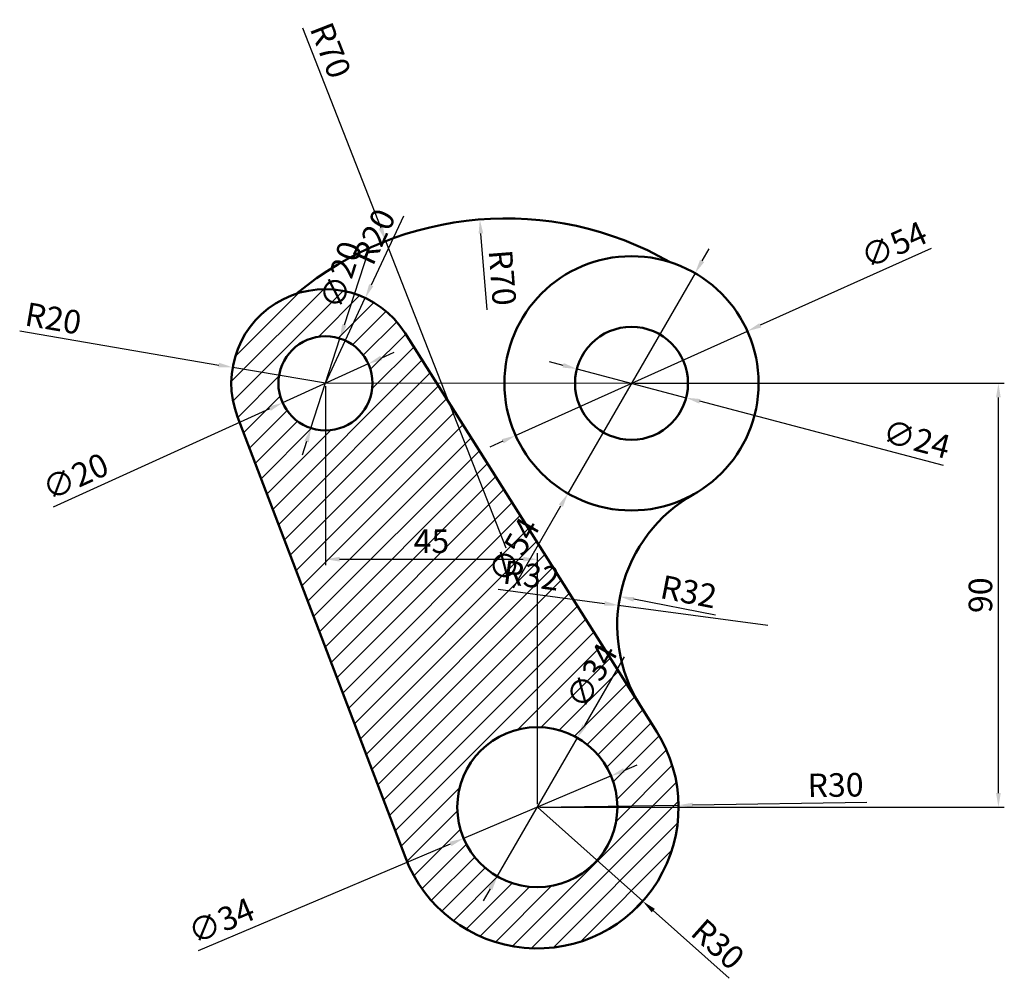
# Model space of a CAD drawing. Units: millimetres. Extents: x 2614 to 2823, y 1450 to 1654.
import ezdxf

# ---------------------------------------------------------------- set-up
doc = ezdxf.new("R2010")
doc.units = ezdxf.units.MM
for name, color, linetype, lineweight in [('M-CONS', 8, 'Continuous', 13), ('M-DIMS', 2, 'Continuous', 25), ('M-HATC', 252, 'Continuous', 18), ('M-OUTL', 7, 'Continuous', 50)]:
    doc.layers.add(name, color=color, linetype=linetype, lineweight=lineweight)
doc.styles.get("Standard").update_dxf_attribs({"font": 'arial.ttf'})
doc.dimstyles.new('ISO-25', dxfattribs={"dimtxt": 5, "dimasz": 3, "dimexe": 1.25, "dimexo": 0.625, "dimtad": 1, "dimtxsty": 'Standard', "dimcen": 3, "dimadec": 0, "dimazin": 0, "dimtfac": 1, "dimtmove": 0, "dimatfit": 3, "dimfxl": 1, "dimarcsym": 0})

# ---------------------------------------------------------------- blocks, each defined once
blk = doc.blocks.new('*D1')
at = {"layer": 'Defpoints', "color": 0, "transparency": 16777216}
for p in [(2739.77, 1493.26), (2708.46, 1480.01)]:
    blk.add_point(p, dxfattribs=at)
at = {"layer": 'M-DIMS', "color": 0, "lineweight": -2, "transparency": 16777216}
for p, q in [((2742.54, 1494.43), (2745.3, 1495.6)), ((2739.77, 1493.26), (2708.46, 1480.01)), ((2652.15, 1456.18), (2705.7, 1478.84))]:
    blk.add_line(p, q, dxfattribs=at)
at = {"layer": 'M-DIMS', "color": 0, "transparency": 16777216}
for points in [[(2742.34, 1494.89), (2742.73, 1493.97), (2739.77, 1493.26)], [(2705.5, 1479.3), (2705.89, 1478.38), (2708.46, 1480.01)]]:
    blk.add_solid(points, dxfattribs=at)
at = {"layer": 'M-DIMS', "color": 0, "transparency": 16777216, "insert": (2657.22, 1461.93), "char_height": 5, "attachment_point": 5, "rotation": 22.939}
blk.add_mtext('∅34', dxfattribs=at)
blk = doc.blocks.new('*D2')
at = {"layer": 'Defpoints', "color": 0, "transparency": 16777216}
for p in [(2688.22, 1580.77), (2670.01, 1572.5)]:
    blk.add_point(p, dxfattribs=at)
at = {"layer": 'M-DIMS', "color": 0, "lineweight": -2, "transparency": 16777216}
for p, q in [((2690.95, 1582.01), (2693.68, 1583.26)), ((2688.22, 1580.77), (2670.01, 1572.5)), ((2621.35, 1550.38), (2667.28, 1571.26))]:
    blk.add_line(p, q, dxfattribs=at)
at = {"layer": 'M-DIMS', "color": 0, "transparency": 16777216}
for points in [[(2690.75, 1582.47), (2691.16, 1581.56), (2688.22, 1580.77)], [(2667.08, 1571.71), (2667.49, 1570.8), (2670.01, 1572.5)]]:
    blk.add_solid(points, dxfattribs=at)
at = {"layer": 'M-DIMS', "color": 0, "transparency": 16777216, "insert": (2626.27, 1556.26), "char_height": 5, "attachment_point": 5, "rotation": 24.4406}
blk.add_mtext('∅20', dxfattribs=at)
blk = doc.blocks.new('*D3')
at = {"layer": 'Defpoints', "color": 0, "transparency": 16777216}
for p in [(2768.74, 1587.72), (2719.5, 1565.55)]:
    blk.add_point(p, dxfattribs=at)
at = {"layer": 'M-DIMS', "color": 0, "lineweight": -2, "transparency": 16777216}
for p, q in [((2807.78, 1605.29), (2771.48, 1588.95)), ((2719.5, 1565.55), (2768.74, 1587.72)), ((2716.76, 1564.32), (2714.02, 1563.09))]:
    blk.add_line(p, q, dxfattribs=at)
at = {"layer": 'M-DIMS', "color": 0, "transparency": 16777216}
for points in [[(2771.27, 1589.4), (2771.68, 1588.49), (2768.74, 1587.72)], [(2716.56, 1564.78), (2716.97, 1563.87), (2719.5, 1565.55)]]:
    blk.add_solid(points, dxfattribs=at)
at = {"layer": 'M-DIMS', "color": 0, "transparency": 16777216, "insert": (2800.11, 1605.47), "char_height": 5, "attachment_point": 5, "rotation": 24.2297}
blk.add_mtext('∅54', dxfattribs=at)
blk = doc.blocks.new('*D4')
at = {"layer": 'Defpoints', "color": 0, "transparency": 16777216}
for p in [(2732.51, 1579.69), (2755.72, 1573.58)]:
    blk.add_point(p, dxfattribs=at)
at = {"layer": 'M-DIMS', "color": 0, "lineweight": -2, "transparency": 16777216}
for p, q in [((2729.61, 1580.45), (2726.71, 1581.22)), ((2732.51, 1579.69), (2755.72, 1573.58)), ((2810.37, 1559.19), (2758.62, 1572.82))]:
    blk.add_line(p, q, dxfattribs=at)
at = {"layer": 'M-DIMS', "color": 0, "transparency": 16777216}
for points in [[(2729.74, 1580.94), (2729.48, 1579.97), (2732.51, 1579.69)], [(2758.75, 1573.3), (2758.5, 1572.33), (2755.72, 1573.58)]]:
    blk.add_solid(points, dxfattribs=at)
at = {"layer": 'M-DIMS', "color": 0, "transparency": 16777216, "insert": (2804.52, 1564.16), "char_height": 5, "attachment_point": 5, "rotation": 345.2499}
blk.add_mtext('∅24', dxfattribs=at)
blk = doc.blocks.new('*D5')
at = {"layer": 'Defpoints', "color": 0, "transparency": 16777216}
for p in [(2754.11, 1487.05), (2724.12, 1486.64)]:
    blk.add_point(p, dxfattribs=at)
at = {"layer": 'M-DIMS', "color": 0, "lineweight": -2, "transparency": 16777216}
for p, q in [((2724.12, 1486.64), (2754.11, 1487.05)), ((2794.1, 1487.6), (2757.11, 1487.09))]:
    blk.add_line(p, q, dxfattribs=at)
at = {"layer": 'M-DIMS', "color": 0, "transparency": 16777216}
blk.add_solid([(2757.11, 1487.59), (2757.12, 1486.59), (2754.11, 1487.05)], dxfattribs=at)
at = {"layer": 'M-DIMS', "color": 0, "transparency": 16777216, "insert": (2787.47, 1490.69), "char_height": 5, "attachment_point": 5, "rotation": 0.7936}
blk.add_mtext('R30', dxfattribs=at)
blk = doc.blocks.new('*D6')
at = {"layer": 'Defpoints', "color": 0, "transparency": 16777216}
for p in [(2659.41, 1580.02), (2679.12, 1576.64)]:
    blk.add_point(p, dxfattribs=at)
at = {"layer": 'M-DIMS', "color": 0, "lineweight": -2, "transparency": 16777216}
for p, q in [((2614.17, 1587.77), (2656.45, 1580.52)), ((2679.12, 1576.64), (2659.41, 1580.02))]:
    blk.add_line(p, q, dxfattribs=at)
at = {"layer": 'M-DIMS', "color": 0, "transparency": 16777216}
blk.add_solid([(2656.53, 1581.01), (2656.36, 1580.03), (2659.41, 1580.02)], dxfattribs=at)
at = {"layer": 'M-DIMS', "color": 0, "transparency": 16777216, "insert": (2621.2, 1589.79), "char_height": 5, "attachment_point": 5, "rotation": 350.2703}
blk.add_mtext('R20', dxfattribs=at)
blk = doc.blocks.new('*D7')
at = {"layer": 'Defpoints', "color": 0, "transparency": 16777216}
for p in [(2711.9, 1611.43), (2717.47, 1541.65)]:
    blk.add_point(p, dxfattribs=at)
at = {"layer": 'M-DIMS', "color": 0, "lineweight": -2, "transparency": 16777216}
blk.add_line((2713.43, 1592.21), (2712.14, 1608.44), dxfattribs=at)
at = {"layer": 'M-DIMS', "color": 0, "transparency": 16777216}
blk.add_solid([(2712.63, 1608.48), (2711.64, 1608.4), (2711.9, 1611.43)], dxfattribs=at)
at = {"layer": 'M-DIMS', "color": 0, "transparency": 16777216, "insert": (2716.07, 1599.03), "char_height": 5, "attachment_point": 5, "rotation": 274.5634}
blk.add_mtext('R70', dxfattribs=at)
blk = doc.blocks.new('*D8')
at = {"layer": 'Defpoints', "color": 0, "transparency": 16777216}
for p in [(2741.66, 1531.34), (2773.07, 1525.23)]:
    blk.add_point(p, dxfattribs=at)
at = {"layer": 'M-DIMS', "color": 0, "lineweight": -2, "transparency": 16777216}
blk.add_line((2761.99, 1527.39), (2744.61, 1530.77), dxfattribs=at)
at = {"layer": 'M-DIMS', "color": 0, "transparency": 16777216}
blk.add_solid([(2744.7, 1531.26), (2744.51, 1530.27), (2741.66, 1531.34)], dxfattribs=at)
at = {"layer": 'M-DIMS', "color": 0, "transparency": 16777216, "insert": (2756.14, 1531.76), "char_height": 5, "attachment_point": 5, "rotation": 348.9946}
blk.add_mtext('R32', dxfattribs=at)
blk = doc.blocks.new('*D9')
at = {"layer": 'Defpoints', "color": 0, "transparency": 16777216}
for p in [(2744.12, 1576.64), (2822.05, 1576.64), (2724.12, 1486.64)]:
    blk.add_point(p, dxfattribs=at)
at = {"layer": 'M-DIMS', "color": 0, "lineweight": -2, "transparency": 16777216}
for p, q in [((2744.74, 1576.64), (2823.3, 1576.64)), ((2822.05, 1489.64), (2822.05, 1573.64)), ((2724.74, 1486.64), (2823.3, 1486.64))]:
    blk.add_line(p, q, dxfattribs=at)
at = {"layer": 'M-DIMS', "color": 0, "transparency": 16777216}
for points in [[(2821.55, 1573.64), (2822.55, 1573.64), (2822.05, 1576.64)], [(2821.55, 1489.64), (2822.55, 1489.64), (2822.05, 1486.64)]]:
    blk.add_solid(points, dxfattribs=at)
at = {"layer": 'M-DIMS', "color": 0, "transparency": 16777216, "insert": (2818.88, 1531.64), "char_height": 5, "attachment_point": 5, "rotation": 90}
blk.add_mtext('90', dxfattribs=at)
blk = doc.blocks.new('*D10')
at = {"layer": 'Defpoints', "color": 0, "transparency": 16777216}
for p in [(2679.12, 1576.64), (2724.12, 1539.29), (2724.12, 1486.64)]:
    blk.add_point(p, dxfattribs=at)
at = {"layer": 'M-DIMS', "color": 0, "lineweight": -2, "transparency": 16777216}
for p, q in [((2679.12, 1576.01), (2679.12, 1538.04)), ((2682.12, 1539.29), (2721.12, 1539.29)), ((2724.12, 1487.26), (2724.12, 1540.54))]:
    blk.add_line(p, q, dxfattribs=at)
at = {"layer": 'M-DIMS', "color": 0, "transparency": 16777216}
for points in [[(2682.12, 1539.79), (2682.12, 1538.79), (2679.12, 1539.29)], [(2721.12, 1539.79), (2721.12, 1538.79), (2724.12, 1539.29)]]:
    blk.add_solid(points, dxfattribs=at)
at = {"layer": 'M-DIMS', "color": 0, "transparency": 16777216, "insert": (2701.62, 1542.46), "char_height": 5, "attachment_point": 5}
blk.add_mtext('45', dxfattribs=at)
blk = doc.blocks.new('*D11')
at = {"layer": 'Defpoints', "color": 0, "transparency": 16777216}
for p in [(2691.96, 1606.84), (2717.47, 1541.65)]:
    blk.add_point(p, dxfattribs=at)
at = {"layer": 'M-DIMS', "color": 0, "lineweight": -2, "transparency": 16777216}
for p, q in [((2674.26, 1652.09), (2690.87, 1609.63)), ((2717.47, 1541.65), (2691.96, 1606.84))]:
    blk.add_line(p, q, dxfattribs=at)
at = {"layer": 'M-DIMS', "color": 0, "transparency": 16777216}
blk.add_solid([(2691.34, 1609.82), (2690.4, 1609.45), (2691.96, 1606.84)], dxfattribs=at)
at = {"layer": 'M-DIMS', "color": 0, "transparency": 16777216, "insert": (2679.62, 1647.11), "char_height": 5, "attachment_point": 5, "rotation": 291.3666}
blk.add_mtext('R70', dxfattribs=at)
blk = doc.blocks.new('*D12')
at = {"layer": 'Defpoints', "color": 0, "transparency": 16777216}
for p in [(2724.12, 1486.64), (2746.51, 1466.67)]:
    blk.add_point(p, dxfattribs=at)
at = {"layer": 'M-DIMS', "color": 0, "lineweight": -2, "transparency": 16777216}
for p, q in [((2724.12, 1486.64), (2746.51, 1466.67)), ((2764.86, 1450.3), (2748.74, 1464.67))]:
    blk.add_line(p, q, dxfattribs=at)
at = {"layer": 'M-DIMS', "color": 0, "transparency": 16777216}
blk.add_solid([(2749.08, 1465.04), (2748.41, 1464.3), (2746.51, 1466.67)], dxfattribs=at)
at = {"layer": 'M-DIMS', "color": 0, "transparency": 16777216, "insert": (2762.05, 1457.06), "char_height": 5, "attachment_point": 5, "rotation": 318.2667}
blk.add_mtext('R30', dxfattribs=at)
blk = doc.blocks.new('*D13')
at = {"layer": 'Defpoints', "color": 0, "transparency": 16777216}
for p in [(2757.62, 1600.02), (2730.62, 1553.25)]:
    blk.add_point(p, dxfattribs=at)
at = {"layer": 'M-DIMS', "color": 0, "lineweight": -2, "transparency": 16777216}
for p, q in [((2759.12, 1602.62), (2760.62, 1605.21)), ((2757.62, 1600.02), (2730.62, 1553.25)), ((2719.06, 1533.23), (2729.12, 1550.65))]:
    blk.add_line(p, q, dxfattribs=at)
at = {"layer": 'M-DIMS', "color": 0, "transparency": 16777216}
for points in [[(2758.68, 1602.87), (2759.55, 1602.37), (2757.62, 1600.02)], [(2728.69, 1550.9), (2729.55, 1550.4), (2730.62, 1553.25)]]:
    blk.add_solid(points, dxfattribs=at)
at = {"layer": 'M-DIMS', "color": 0, "transparency": 16777216, "insert": (2719.65, 1540.88), "char_height": 5, "attachment_point": 5, "rotation": 60.0007}
blk.add_mtext('∅54', dxfattribs=at)
blk = doc.blocks.new('*D14')
at = {"layer": 'Defpoints', "color": 0, "transparency": 16777216}
for p in [(2687.57, 1594.76), (2679.12, 1576.64)]:
    blk.add_point(p, dxfattribs=at)
at = {"layer": 'M-DIMS', "color": 0, "lineweight": -2, "transparency": 16777216}
for p, q in [((2695.68, 1612.14), (2688.84, 1597.48)), ((2679.12, 1576.64), (2687.57, 1594.76))]:
    blk.add_line(p, q, dxfattribs=at)
at = {"layer": 'M-DIMS', "color": 0, "transparency": 16777216}
blk.add_solid([(2688.39, 1597.69), (2689.29, 1597.27), (2687.57, 1594.76)], dxfattribs=at)
at = {"layer": 'M-DIMS', "color": 0, "transparency": 16777216, "insert": (2690.01, 1607.51), "char_height": 5, "attachment_point": 5, "rotation": 64.999}
blk.add_mtext('R20', dxfattribs=at)
blk = doc.blocks.new('*D15')
at = {"layer": 'Defpoints', "color": 0, "transparency": 16777216}
for p in [(2732.62, 1501.36), (2715.62, 1471.91)]:
    blk.add_point(p, dxfattribs=at)
at = {"layer": 'M-DIMS', "color": 0, "lineweight": -2, "transparency": 16777216}
for p, q in [((2742.53, 1518.53), (2734.12, 1503.96)), ((2715.62, 1471.91), (2732.62, 1501.36)), ((2714.12, 1469.31), (2712.62, 1466.72))]:
    blk.add_line(p, q, dxfattribs=at)
at = {"layer": 'M-DIMS', "color": 0, "transparency": 16777216}
for points in [[(2733.69, 1504.21), (2734.55, 1503.71), (2732.62, 1501.36)], [(2713.68, 1469.56), (2714.55, 1469.06), (2715.62, 1471.91)]]:
    blk.add_solid(points, dxfattribs=at)
at = {"layer": 'M-DIMS', "color": 0, "transparency": 16777216, "insert": (2736.2, 1514.2), "char_height": 5, "attachment_point": 5, "rotation": 59.9979}
blk.add_mtext('∅34', dxfattribs=at)
blk = doc.blocks.new('*D16')
at = {"layer": 'Defpoints', "color": 0, "transparency": 16777216}
for p in [(2682.2, 1586.15), (2676.04, 1567.12)]:
    blk.add_point(p, dxfattribs=at)
at = {"layer": 'M-DIMS', "color": 0, "lineweight": -2, "transparency": 16777216}
for p, q in [((2688.31, 1605.02), (2683.12, 1589)), ((2676.04, 1567.12), (2682.2, 1586.15)), ((2675.11, 1564.27), (2674.19, 1561.41))]:
    blk.add_line(p, q, dxfattribs=at)
at = {"layer": 'M-DIMS', "color": 0, "transparency": 16777216}
for points in [[(2682.65, 1589.16), (2683.6, 1588.85), (2682.2, 1586.15)], [(2674.64, 1564.42), (2675.59, 1564.11), (2676.04, 1567.12)]]:
    blk.add_solid(points, dxfattribs=at)
at = {"layer": 'M-DIMS', "color": 0, "transparency": 16777216, "insert": (2683.02, 1599.46), "char_height": 5, "attachment_point": 5, "rotation": 72.0514}
blk.add_mtext('∅20', dxfattribs=at)
blk = doc.blocks.new('*D17')
at = {"layer": 'Defpoints', "color": 0, "transparency": 16777216}
for p in [(2741.36, 1529.49), (2773.07, 1525.23)]:
    blk.add_point(p, dxfattribs=at)
at = {"layer": 'M-DIMS', "color": 0, "lineweight": -2, "transparency": 16777216}
for p, q in [((2715.82, 1532.92), (2738.39, 1529.89)), ((2773.07, 1525.23), (2741.36, 1529.49))]:
    blk.add_line(p, q, dxfattribs=at)
at = {"layer": 'M-DIMS', "color": 0, "transparency": 16777216}
blk.add_solid([(2738.45, 1530.39), (2738.32, 1529.39), (2741.36, 1529.49)], dxfattribs=at)
at = {"layer": 'M-DIMS', "color": 0, "transparency": 16777216, "insert": (2722.75, 1535.2), "char_height": 5, "attachment_point": 5, "rotation": 352.3473}
blk.add_mtext('R32', dxfattribs=at)

msp = doc.modelspace()

# ---------------------------------------------------------------- hatches: boundary and pattern name
at = {"layer": 'M-HATC'}
h = msp.add_hatch(dxfattribs=at)
h.set_pattern_fill('ANSI31', color=256)
h.paths.add_polyline_path([(2702.771, 1576.635), (2689.118, 1576.635, -1), (2669.118, 1576.635, -1), (2689.118, 1576.635), (2702.771, 1576.635), (2696.029, 1587.313, 0.9050999), (2660.429, 1569.513), (2696.085, 1475.952, 1.1048504), (2749.484, 1502.652)])
h.paths.add_polyline_path([(2741.118, 1486.635, -1), (2707.118, 1486.635, -1)], flags=16)
h.paths.add_polyline_path([(2696.579, 1537.269), (2706.848, 1537.269), (2706.848, 1547.572), (2696.579, 1547.572)], flags=24)

# ---------------------------------------------------------------- linework, layer by layer
at = {"layer": 'M-CONS'}
msp.add_line((2679.118, 1576.635), (2744.118, 1576.635), dxfattribs=at)
at = {"layer": 'M-OUTL'}
for p, q in [((2696.029, 1587.313), (2749.484, 1502.652)), ((2660.429, 1569.513), (2696.085, 1475.952)), ((2746.016, 1508.145), (2749.484, 1502.652))]:
    msp.add_line(p, q, dxfattribs=at)
for centre, radius in [((2744.118, 1576.635), 27), ((2744.118, 1576.635), 12), ((2679.118, 1576.635), 10), ((2724.118, 1486.635), 17)]:
    msp.add_circle(centre, radius, dxfattribs=at)
for centre, radius, start, end in [((2717.466, 1541.652), 70, 60.14427, 129.51729), ((2679.118, 1576.635), 20, 32.26857, 200.86154), ((2773.074, 1525.229), 32, 119.39182, 212.26857), ((2724.118, 1486.635), 30, 200.86154, 32.26857)]:
    msp.add_arc(centre, radius, start, end, dxfattribs=at)

# ---------------------------------------------------------------- dimensions: what is measured, and where the dimension line sits
at = {"layer": 'M-DIMS'}
for center, mpoint, override, picture, middle in [((2717.466, 1541.652), (2691.962, 1606.84), {"dimdec": 0, "dimlfac": 1, "dimrnd": 0, "dimzin": 0, "dimdsep": 46, "dimlunit": 2}, '*D11', (2676.66, 1645.954)), ((2717.466, 1541.652), (2711.896, 1611.43), {"dimclrd": 0, "dimclre": 0, "dimclrt": 0}, '*D7', (2712.906, 1598.776)), ((2679.118, 1576.635), (2659.406, 1580.015), {"dimclrd": 0, "dimclre": 0, "dimclrt": 0}, '*D6', (2620.664, 1586.658)), ((2773.074, 1525.229), (2741.359, 1529.491), {"dimdec": 0, "dimlfac": 1, "dimrnd": 0, "dimzin": 0, "dimdsep": 46, "dimlunit": 2}, '*D17', (2722.33, 1532.048)), ((2773.074, 1525.229), (2741.662, 1531.338), {"dimclrd": 0, "dimclre": 0, "dimclrt": 0}, '*D8', (2755.537, 1528.64)), ((2724.118, 1486.635), (2754.115, 1487.051), {"dimclrd": 0, "dimclre": 0, "dimclrt": 0}, '*D5', (2787.509, 1487.513)), ((2724.118, 1486.635), (2746.505, 1466.665), {"dimdec": 0, "dimlfac": 1, "dimrnd": 0, "dimzin": 0, "dimdsep": 46, "dimlunit": 2}, '*D12', (2759.938, 1454.683))]:
    dim = msp.add_radius_dim(center=center, mpoint=mpoint, dimstyle='ISO-25', override=override, dxfattribs=at)
    dim.commit()
    dim.dimension.update_dxf_attribs({"geometry": picture, "text_midpoint": middle, "dimtype": 164})
dim = msp.add_radius_dim(center=(2679.118, 1576.635), mpoint=(2687.571, 1594.761), dimstyle='ISO-25', override={"dimdec": 0, "dimlfac": 1, "dimrnd": 0, "dimzin": 0, "dimdsep": 46, "dimlunit": 2}, dxfattribs=at)
dim.commit()
dim.dimension.update_dxf_attribs({"geometry": '*D14', "text_midpoint": (2690.011, 1607.515)})
for p1, p2, override, picture, middle in [((2719.496, 1565.554), (2768.739, 1587.716), {"dimclrd": 0, "dimclre": 0, "dimclrt": 0}, '*D3', (2801.474, 1602.448)), ((2676.036, 1567.122), (2682.199, 1586.148), {"dimdec": 0, "dimlfac": 1, "dimrnd": 0, "dimzin": 0, "dimdsep": 46, "dimlunit": 2}, '*D16', (2686.18, 1598.437)), ((2757.618, 1600.018), (2730.618, 1553.252), {"dimdec": 0, "dimlfac": 1, "dimrnd": 0, "dimzin": 0, "dimdsep": 46, "dimlunit": 2}, '*D13', (2722.518, 1539.223)), ((2688.222, 1580.773), (2670.014, 1572.498), {"dimclrd": 0, "dimclre": 0, "dimclrt": 0}, '*D2', (2627.646, 1553.243)), ((2732.513, 1579.69), (2755.722, 1573.58), {"dimclrd": 0, "dimclre": 0, "dimclrt": 0}, '*D4', (2803.679, 1560.954)), ((2739.774, 1493.261), (2708.462, 1480.009), {"dimclrd": 0, "dimclre": 0, "dimclrt": 0}, '*D1', (2658.516, 1458.871))]:
    dim = msp.add_diameter_dim_2p(p1=p1, p2=p2, dimstyle='ISO-25', override=override, dxfattribs=at)
    dim.commit()
    dim.dimension.update_dxf_attribs({"geometry": picture, "text_midpoint": middle, "dimtype": 163})
dim = msp.add_linear_dim(base=(2724.118, 1539.289), p1=(2679.118, 1576.635), p2=(2724.118, 1486.635), dimstyle='ISO-25', override={"dimclrd": 0, "dimclre": 0, "dimclrt": 0}, dxfattribs=at)
dim.commit()
dim.dimension.update_dxf_attribs({"geometry": '*D10', "text_midpoint": (2701.618, 1542.456)})
dim = msp.add_linear_dim(base=(2822.054, 1576.635), p1=(2724.118, 1486.635), p2=(2744.118, 1576.635), angle=90, dimstyle='ISO-25', override={"dimclrd": 0, "dimclre": 0, "dimclrt": 0}, dxfattribs=at)
dim.commit()
dim.dimension.update_dxf_attribs({"geometry": '*D9', "text_midpoint": (2818.876, 1531.635)})
dim = msp.add_diameter_dim_2p(p1=(2715.617, 1471.913), p2=(2732.618, 1501.357), dimstyle='ISO-25', override={"dimdec": 0, "dimlfac": 1, "dimrnd": 0, "dimzin": 0, "dimdsep": 46, "dimlunit": 2}, dxfattribs=at)
dim.commit()
dim.dimension.update_dxf_attribs({"geometry": '*D15', "text_midpoint": (2739.077, 1512.542)})

doc.saveas('drawing.dxf')
